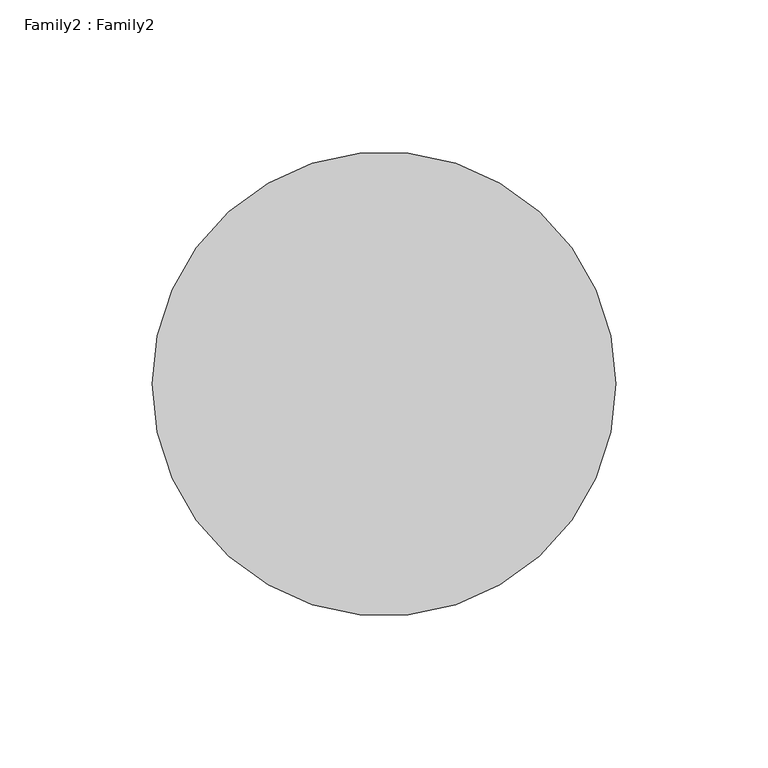
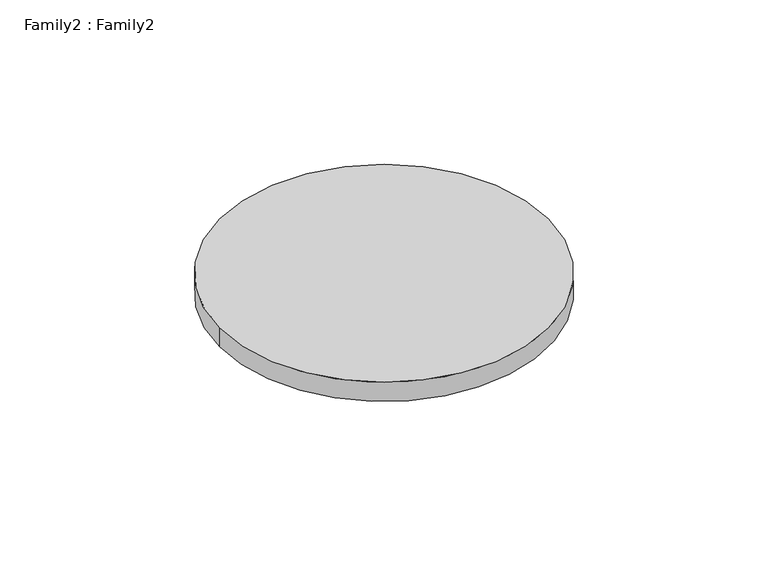
"""IFC4 building model written with IfcOpenShell, lengths in millimetres: light fixture geometry, Family2 : Family2."""

from ifc_helpers import new_model, si_unit, point, frame, origin, origin_2d, place, context, project, spatial, circle_curve, trimmed, segment, composite_curve, outline, extrude, source, transform, mapped, element, save


def family2_family2_8c2629c1(model_context):
    return source(origin(), model_context, "Body", "SweptSolid", [
        extrude(outline(composite_curve([segment(trimmed(circle_curve(origin_2d(), 76.2), [point((-76.2, 0.0))], [point((76.2, 0.0))], False, "CARTESIAN"), True, "CONTINUOUS"), segment(trimmed(circle_curve(origin_2d(), 76.2), [point((76.2, 0.0))], [point((-76.2, 0.0))], False, "CARTESIAN"), True, "CONTINUOUS")], self_intersect=False)), frame((0.0, 0.0, 2541.3376221), z_axis=(0.0, 0.0, 1.0), x_axis=(1.0, 0.0, 0.0)), (0.0, 0.0, 1.0), 9.3724029),
    ])


if __name__ == "__main__":
    model = new_model("IFC4")
    model_context = context("Model", 3, world=origin())
    ifc_project = project(units=[si_unit("LENGTHUNIT", "METRE", prefix="MILLI")], contexts=[model_context])
    site = spatial("IfcSite", under=ifc_project)
    building = spatial("IfcBuilding", under=site)
    placement = place(None, origin())
    family2_family2_shape = family2_family2_8c2629c1(model_context)
    element("IfcLightFixture", 1, ObjectType="Family2 : Family2", at=placement, inside=building, context=model_context, shape_type="MappedRepresentation", body=[
        mapped(family2_family2_shape, transform((0.0, 0.0, 0.0), x_axis=(1.0, 0.0, 0.0), y_axis=(0.0, 1.0, 0.0), z_axis=(0.0, 0.0, 1.0))),
    ])
    save(model, "model.ifc")

# Revit data of these elements
# Type "Family2 : Family2"
#   Wattage = 27 W
#   built-in parameter 1150110 = 1 (stored number, unit not read)
#   built-in parameter 1114217 = 1 (stored number, unit not read)
#   built-in parameter 1150109 = 1 (stored number, unit not read)
#   built-in parameter 1150113 = 1 (stored number, unit not read)
#   Lumens = 4010.63 lm
#   built-in parameter 1150115 = 1 (stored number, unit not read)
#   built-in parameter 1150105 = 319.156 (stored number, unit not read)
#   Light Source Symbol Size = 2' - 0"
#   built-in parameter 1150112 = 1 (stored number, unit not read)
#   built-in parameter 1150114 = 1 (stored number, unit not read)
#   built-in parameter 1150107 = 3000 (stored number, unit not read)
#   built-in parameter 1150106 = 3.19156 (stored number, unit not read)
#   built-in parameter 1150104 = 13.8 (stored number, unit not read)
#   built-in parameter 1114218 = 1 (stored number, unit not read)
#   built-in parameter 1150133 = 10 (stored number, unit not read)
#   Color Filter = 16777215
#   Dimming Lamp Color Temperature Shift = (empty or 0)
#   Default Elevation = 0
